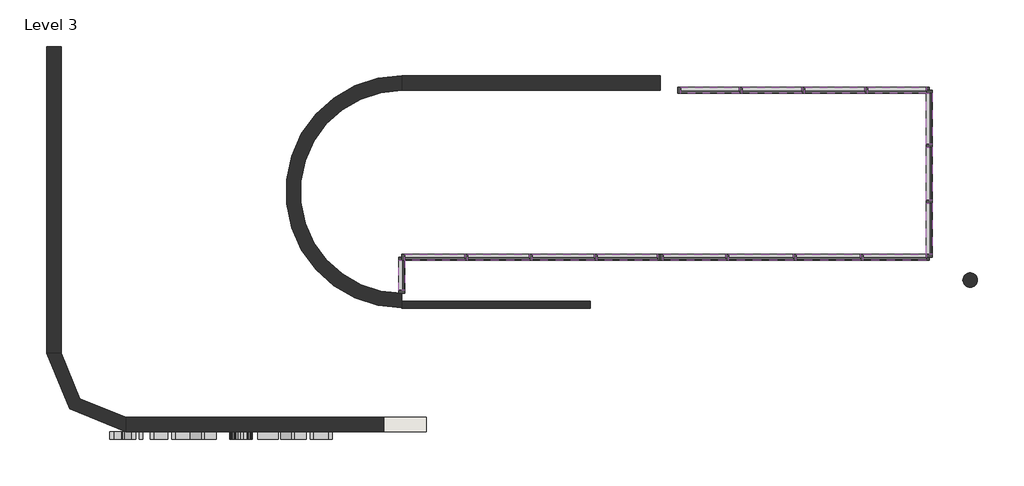
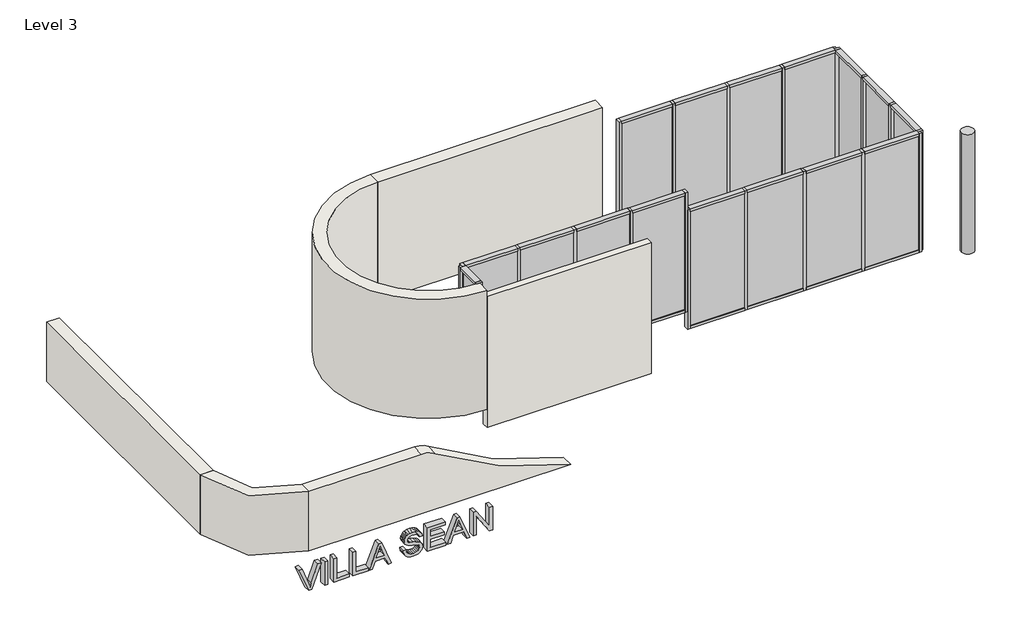
# One storey: 53 members, 16 plates, 6 walls, 1 column, 1 proxy.
"""IFC4 building model written with IfcOpenShell, lengths in millimetres."""

from ifc_helpers import new_model, si_unit, point, frame, frame_2d, origin, place, context, project, spatial, polyline, circle_curve, trimmed, segment, composite_curve, outline, extrude, transform, mapped, element, save
from components import column_6a8e800d, member_4d6ef9b1, member_8897803d, member_ef344e51, member_b14cf619, member_0d684f40, member_efa17701, member_5e365d0c, member_eaba9652, member_3f395ae9, member_5a365947, member_16d8dc0e, system_panel_glazed_93f0cbb4, system_panel_glazed_f623c012, system_panel_glazed_38c921e2, system_panel_glazed_90a2254b, system_panel_glazed_fd2dabf8, system_panel_glazed_5b6ff290, system_panel_glazed_14fb9695, system_panel_glazed_f99b9bb8, system_panel_glazed_f492b607

model = new_model("IFC4")

# Units and contexts
model_context = context("Model", 3, world=origin())
ifc_project = project(units=[si_unit("LENGTHUNIT", "METRE", prefix="MILLI")], contexts=[model_context])

# Site, building, storey
site = spatial("IfcSite", under=ifc_project)
building = spatial("IfcBuilding", under=site)
storey = spatial("IfcBuildingStorey", under=building, Name="Level 3", Elevation=6096.0)

# Proxy
placement = place(None, origin())
element("IfcBuildingElementProxy", 1, Name="24\" Arial", ObjectType="24\" Arial", at=placement, inside=storey, context=model_context, shape_type="SweptSolid", body=[
    extrude(outline(polyline([(6126.8228515, -15529.5610771), (6126.8228515, -15452.1887694), (6727.0443899, -15223.2956925), (6727.0443899, -15303.452231), (6294.6093899, -15463.7653079), (6197.161313, -15495.7106925), (6294.6093899, -15528.0956925), (6727.0443899, -15687.969154), (6727.0443899, -15768.272231), (6126.8228515, -15529.5610771)])), frame((0.0, 6721.4139644, 0.0), z_axis=(0.0, 1.0, 0.0), x_axis=(0.0, 0.0, 1.0)), (0.0, 0.0, 1.0), 152.4),
    extrude(outline(polyline([(-15068.9906925, 6721.4139644), (-15144.0183848, 6721.4139644), (-15144.0183848, 6873.8139644), (-15068.9906925, 6873.8139644), (-15068.9906925, 6721.4139644)])), frame((0.0, 0.0, 6126.8228515), z_axis=(0.0, 0.0, 1.0), x_axis=(1.0, 0.0, 0.0)), (0.0, 0.0, 1.0), 600.2215385),
    extrude(outline(polyline([(6126.8228515, -14918.9353079), (6126.8228515, -14543.7968463), (6201.8505438, -14543.7968463), (6201.8505438, -14843.9076156), (6727.0443899, -14843.9076156), (6727.0443899, -14918.9353079), (6126.8228515, -14918.9353079)])), frame((0.0, 6721.4139644, 0.0), z_axis=(0.0, 1.0, 0.0), x_axis=(0.0, 0.0, 1.0)), (0.0, 0.0, 1.0), 152.4),
    extrude(outline(polyline([(6126.8228515, -14459.3906925), (6126.8228515, -14084.252231), (6201.8505438, -14084.252231), (6201.8505438, -14384.3630002), (6727.0443899, -14384.3630002), (6727.0443899, -14459.3906925), (6126.8228515, -14459.3906925)])), frame((0.0, 6721.4139644, 0.0), z_axis=(0.0, 1.0, 0.0), x_axis=(0.0, 0.0, 1.0)), (0.0, 0.0, 1.0), 152.4),
    extrude(outline(polyline([(6126.8228515, -14069.5983848), (6126.8228515, -13990.4676156), (6314.3920822, -13921.8876156), (6314.3920822, -13674.5306925), (6126.8228515, -13605.9506925), (6126.8228515, -13526.6733848), (6727.0443899, -13766.117231), (6727.0443899, -13830.0080002), (6126.8228515, -14069.5983848)]), holes=[polyline([(6389.4197745, -13894.3383848), (6549.8793899, -13835.5764617), (6652.0166976, -13798.209154), (6536.9840053, -13756.1526156), (6389.4197745, -13701.9333848), (6389.4197745, -13894.3383848)])]), frame((0.0, 6721.4139644, 0.0), z_axis=(0.0, 1.0, 0.0), x_axis=(0.0, 0.0, 1.0)), (0.0, 0.0, 1.0), 152.4),
    extrude(outline(polyline([(6333.1490053, -13240.1906925), (6302.0278995, -13237.5621588), (6272.5553515, -13231.288481), (6244.7313611, -13221.3696588), (6218.5559284, -13207.8056925), (6194.7983803, -13190.9675074), (6174.2280438, -13171.226029), (6156.8449188, -13148.5812574), (6142.6490053, -13123.0331925), (6131.6219861, -13094.4078199), (6123.7455438, -13062.5311252), (6119.0196784, -13027.4031084), (6117.4443899, -12989.0237694), (6123.2876111, -12929.1444906), (6130.5916375, -12901.5540459), (6140.8172745, -12875.529731), (6153.6760245, -12851.7630242), (6168.8793899, -12830.945404), (6186.4273707, -12813.0768704), (6206.3199668, -12798.1574233), (6227.7283202, -12786.3931324), (6249.8235726, -12777.9900675), (6272.605724, -12772.9482286), (6296.0747745, -12771.2676156), (6341.3185245, -12777.1108367), (6361.8247505, -12784.4148632), (6380.9205438, -12794.6405002), (6398.5143178, -12807.9434449), (6414.5144861, -12824.4793944), (6441.7340053, -12867.2503079), (6459.2819861, -12917.2931925), (6479.3943899, -13000.014154), (6500.5691976, -13080.1706925), (6510.9917457, -13106.0713656), (6521.3043899, -13122.5203079), (6532.1940293, -13132.9703319), (6544.4941015, -13140.4346348), (6558.2046063, -13144.9132165), (6573.3255438, -13146.4060771), (6590.9010005, -13144.2995867), (6607.1392938, -13137.9801156), (6622.0404236, -13127.4476637), (6635.6043899, -13112.702231), (6646.8878515, -13093.3499954), (6654.9474668, -13068.9971348), (6659.7832361, -13039.6436492), (6661.3951591, -13005.2895387), (6659.7649188, -12971.9978319), (6654.8741976, -12943.0473271), (6646.7229957, -12918.4380242), (6635.311313, -12898.1699233), (6620.7124188, -12881.9407887), (6602.9995822, -12869.4483848), (6582.1728034, -12860.6927117), (6558.2320822, -12855.6737694), (6558.2320822, -12780.6460771), (6583.7755678, -12783.2746108), (6607.9452553, -12789.1086733), (6630.7411447, -12798.1482646), (6652.1632361, -12810.3933848), (6671.6436928, -12825.7249713), (6688.6146784, -12844.0239617), (6703.0761928, -12865.290356), (6715.0282361, -12889.524154), (6731.0741976, -12944.9156925), (6736.4228515, -13008.2203079), (6731.3123226, -13066.6525194), (6715.9807361, -13119.4430002), (6704.5690534, -13142.930368), (6690.7761207, -13163.422856), (6674.601938, -13180.9204641), (6656.0465053, -13195.4231925), (6635.9295221, -13206.8028199), (6615.070688, -13214.9311252), (6593.4700029, -13219.8081084), (6571.1274668, -13221.4337694), (6531.8185245, -13216.1767021), (6496.5393899, -13200.4055002), (6465.9494861, -13173.9369906), (6440.7082361, -13136.5880002), (6422.665688, -13090.7031444), (6403.7072745, -13018.9908848), (6375.0590053, -12909.7464617), (6359.5076111, -12877.7278079), (6340.988813, -12858.7510771), (6319.2828034, -12849.4092502), (6294.1697745, -12846.2953079), (6268.3973226, -12850.4533367), (6243.833813, -12862.9274233), (6222.4391976, -12883.9007406), (6206.1734284, -12913.5564617), (6195.8974188, -12950.1544425), (6192.4720822, -12991.9545387), (6196.9964572, -13039.4330002), (6210.5695822, -13081.929154), (6231.4879476, -13116.695404), (6258.0480438, -13140.984154), (6291.5137649, -13156.5538656), (6333.1490053, -13165.1630002), (6333.1490053, -13240.1906925)])), frame((0.0, 6721.4139644, 0.0), z_axis=(0.0, 1.0, 0.0), x_axis=(0.0, 0.0, 1.0)), (0.0, 0.0, 1.0), 152.4),
    extrude(outline(polyline([(6126.8228515, -12658.7260771), (6126.8228515, -12217.9383848), (6201.8505438, -12217.9383848), (6201.8505438, -12583.6983848), (6398.7982361, -12583.6983848), (6398.7982361, -12246.0737694), (6473.8259284, -12246.0737694), (6473.8259284, -12583.6983848), (6652.0166976, -12583.6983848), (6652.0166976, -12227.3168463), (6727.0443899, -12227.3168463), (6727.0443899, -12658.7260771), (6126.8228515, -12658.7260771)])), frame((0.0, 6721.4139644, 0.0), z_axis=(0.0, 1.0, 0.0), x_axis=(0.0, 0.0, 1.0)), (0.0, 0.0, 1.0), 152.4),
    extrude(outline(polyline([(6126.8228515, -12175.149154), (6126.8228515, -12096.0183848), (6314.3920822, -12027.4383848), (6314.3920822, -11780.0814617), (6126.8228515, -11711.5014617), (6126.8228515, -11632.224154), (6727.0443899, -11871.6680002), (6727.0443899, -11935.5587694), (6126.8228515, -12175.149154)]), holes=[polyline([(6389.4197745, -11999.889154), (6549.8793899, -11941.127231), (6652.0166976, -11903.7599233), (6536.9840053, -11861.7033848), (6389.4197745, -11807.484154), (6389.4197745, -11999.889154)])]), frame((0.0, 6721.4139644, 0.0), z_axis=(0.0, 1.0, 0.0), x_axis=(0.0, 0.0, 1.0)), (0.0, 0.0, 1.0), 152.4),
    extrude(outline(polyline([(6126.8228515, -11552.0676156), (6126.8228515, -11477.0399233), (6602.4866976, -11477.0399233), (6126.8228515, -11163.4476156), (6126.8228515, -11083.1445387), (6727.0443899, -11083.1445387), (6727.0443899, -11158.172231), (6251.5270822, -11158.172231), (6727.0443899, -11471.7645387), (6727.0443899, -11552.0676156), (6126.8228515, -11552.0676156)])), frame((0.0, 6721.4139644, 0.0), z_axis=(0.0, 1.0, 0.0), x_axis=(0.0, 0.0, 1.0)), (0.0, 0.0, 1.0), 152.4),
])

# Column
column_shape = column_6a8e800d(model_context)
element("IfcColumn", 2, ObjectType="Round Column.0002 : 06\" Diameter", at=placement, inside=storey, context=model_context, shape_type="MappedRepresentation", body=[
    mapped(column_shape, transform((-1667.0944013, 3216.2139644, 0.0), x_axis=(1.0, 0.0, 0.0), y_axis=(0.0, 1.0, 0.0), z_axis=(0.0, 0.0, 1.0))),
])

# Members
member_shape = member_4d6ef9b1(model_context)
element("IfcMember", 3, ObjectType="Rectangular Mullion : 2.5\" x 5\" rectangular", at=placement, inside=storey, context=model_context, shape_type="MappedRepresentation", body=[
    mapped(member_shape, transform((1468.8829427, 10615.9053975, 9601.2), x_axis=(0.0, 0.0, 1.0), y_axis=(-1.0, 0.0, 0.0), z_axis=(0.0, -1.0, 0.0))),
])
element("IfcMember", 4, ObjectType="Rectangular Mullion : 2.5\" x 5\" rectangular", at=placement, inside=storey, context=model_context, shape_type="MappedRepresentation", body=[
    mapped(member_shape, transform((1468.8829427, 12920.9553975, 9601.2), x_axis=(0.0, 0.0, 1.0), y_axis=(-1.0, 0.0, 0.0), z_axis=(0.0, -1.0, 0.0))),
])
member_2_shape = member_8897803d(model_context)
element("IfcMember", 5, ObjectType="Rectangular Mullion : 2.5\" x 5\" rectangular", at=placement, inside=storey, context=model_context, shape_type="MappedRepresentation", body=[
    mapped(member_2_shape, transform((1468.8829427, 11752.5553975, 9601.2), x_axis=(0.0, 0.0, 1.0), y_axis=(-1.0, 0.0, 0.0), z_axis=(0.0, -1.0, 0.0))),
])
element("IfcMember", 6, ObjectType="Rectangular Mullion : 2.5\" x 5\" rectangular", at=placement, inside=storey, context=model_context, shape_type="MappedRepresentation", body=[
    mapped(member_shape, transform((1468.8829427, 13994.1053975, 6553.2), x_axis=(0.0, 0.0, -1.0), y_axis=(-1.0, 0.0, 0.0), z_axis=(0.0, 1.0, 0.0))),
])
element("IfcMember", 7, ObjectType="Rectangular Mullion : 2.5\" x 5\" rectangular", at=placement, inside=storey, context=model_context, shape_type="MappedRepresentation", body=[
    mapped(member_shape, transform((1468.8829427, 11689.0553975, 6553.2), x_axis=(0.0, 0.0, -1.0), y_axis=(-1.0, 0.0, 0.0), z_axis=(0.0, 1.0, 0.0))),
])
element("IfcMember", 8, ObjectType="Rectangular Mullion : 2.5\" x 5\" rectangular", at=placement, inside=storey, context=model_context, shape_type="MappedRepresentation", body=[
    mapped(member_2_shape, transform((1468.8829427, 12857.4553975, 6553.2), x_axis=(0.0, 0.0, -1.0), y_axis=(-1.0, 0.0, 0.0), z_axis=(0.0, 1.0, 0.0))),
])
member_3_shape = member_ef344e51(model_context)
element("IfcMember", 9, ObjectType="Rectangular Mullion : 2.5\" x 5\" rectangular", at=placement, inside=storey, context=model_context, shape_type="MappedRepresentation", body=[
    mapped(member_3_shape, transform((-4128.3438771, 10552.4053975, 9601.2), x_axis=(0.0, 0.0, 1.0), y_axis=(0.0, 1.0, 0.0), z_axis=(-1.0, 0.0, 0.0))),
])
element("IfcMember", 10, ObjectType="Rectangular Mullion : 2.5\" x 5\" rectangular", at=placement, inside=storey, context=model_context, shape_type="MappedRepresentation", body=[
    mapped(member_3_shape, transform((85.4512378, 10552.4053975, 9601.2), x_axis=(0.0, 0.0, 1.0), y_axis=(0.0, 1.0, 0.0), z_axis=(-1.0, 0.0, 0.0))),
])
member_4_shape = member_b14cf619(model_context)
element("IfcMember", 11, ObjectType="Rectangular Mullion : 2.5\" x 5\" rectangular", at=placement, inside=storey, context=model_context, shape_type="MappedRepresentation", body=[
    mapped(member_4_shape, transform((-1329.7304672, 10552.4053975, 9601.2), x_axis=(0.0, 0.0, 1.0), y_axis=(0.0, 1.0, 0.0), z_axis=(-1.0, 0.0, 0.0))),
])
element("IfcMember", 12, ObjectType="Rectangular Mullion : 2.5\" x 5\" rectangular", at=placement, inside=storey, context=model_context, shape_type="MappedRepresentation", body=[
    mapped(member_4_shape, transform((-2744.9121722, 10552.4053975, 9601.2), x_axis=(0.0, 0.0, 1.0), y_axis=(0.0, 1.0, 0.0), z_axis=(-1.0, 0.0, 0.0))),
])
element("IfcMember", 13, ObjectType="Rectangular Mullion : 2.5\" x 5\" rectangular", at=placement, inside=storey, context=model_context, shape_type="MappedRepresentation", body=[
    mapped(member_3_shape, transform((1405.3829427, 10552.4053975, 6553.2), x_axis=(0.0, 0.0, -1.0), y_axis=(0.0, 1.0, 0.0), z_axis=(1.0, 0.0, 0.0))),
])
element("IfcMember", 14, ObjectType="Rectangular Mullion : 2.5\" x 5\" rectangular", at=placement, inside=storey, context=model_context, shape_type="MappedRepresentation", body=[
    mapped(member_3_shape, transform((-2808.4121722, 10552.4053975, 6553.2), x_axis=(0.0, 0.0, -1.0), y_axis=(0.0, 1.0, 0.0), z_axis=(1.0, 0.0, 0.0))),
])
element("IfcMember", 15, ObjectType="Rectangular Mullion : 2.5\" x 5\" rectangular", at=placement, inside=storey, context=model_context, shape_type="MappedRepresentation", body=[
    mapped(member_4_shape, transform((21.9512378, 10552.4053975, 6553.2), x_axis=(0.0, 0.0, -1.0), y_axis=(0.0, 1.0, 0.0), z_axis=(1.0, 0.0, 0.0))),
])
element("IfcMember", 16, ObjectType="Rectangular Mullion : 2.5\" x 5\" rectangular", at=placement, inside=storey, context=model_context, shape_type="MappedRepresentation", body=[
    mapped(member_4_shape, transform((-1393.2304672, 10552.4053975, 6553.2), x_axis=(0.0, 0.0, -1.0), y_axis=(0.0, 1.0, 0.0), z_axis=(1.0, 0.0, 0.0))),
])
member_5_shape = member_0d684f40(model_context)
element("IfcMember", 17, ObjectType="Rectangular Mullion : 2.5\" x 5\" rectangular", at=placement, inside=storey, context=model_context, shape_type="MappedRepresentation", body=[
    mapped(member_5_shape, transform((-9560.164807, 10552.4053975, 10058.4), x_axis=(0.0, 0.0, 1.0), y_axis=(0.0, 1.0, 0.0), z_axis=(-1.0, 0.0, 0.0))),
])
element("IfcMember", 18, ObjectType="Rectangular Mullion : 2.5\" x 5\" rectangular", at=placement, inside=storey, context=model_context, shape_type="MappedRepresentation", body=[
    mapped(member_5_shape, transform((-5518.0491096, 10552.4053975, 10058.4), x_axis=(0.0, 0.0, 1.0), y_axis=(0.0, 1.0, 0.0), z_axis=(-1.0, 0.0, 0.0))),
])
member_6_shape = member_efa17701(model_context)
element("IfcMember", 19, ObjectType="Rectangular Mullion : 2.5\" x 5\" rectangular", at=placement, inside=storey, context=model_context, shape_type="MappedRepresentation", body=[
    mapped(member_6_shape, transform((-6876.004342, 10552.4053975, 10058.4), x_axis=(0.0, 0.0, 1.0), y_axis=(0.0, 1.0, 0.0), z_axis=(-1.0, 0.0, 0.0))),
])
element("IfcMember", 20, ObjectType="Rectangular Mullion : 2.5\" x 5\" rectangular", at=placement, inside=storey, context=model_context, shape_type="MappedRepresentation", body=[
    mapped(member_6_shape, transform((-8233.9595745, 10552.4053975, 10058.4), x_axis=(0.0, 0.0, 1.0), y_axis=(0.0, 1.0, 0.0), z_axis=(-1.0, 0.0, 0.0))),
])
element("IfcMember", 21, ObjectType="Rectangular Mullion : 2.5\" x 5\" rectangular", at=placement, inside=storey, context=model_context, shape_type="MappedRepresentation", body=[
    mapped(member_5_shape, transform((-4255.3438771, 10552.4053975, 7010.4), x_axis=(0.0, 0.0, -1.0), y_axis=(0.0, 1.0, 0.0), z_axis=(1.0, 0.0, 0.0))),
])
element("IfcMember", 22, ObjectType="Rectangular Mullion : 2.5\" x 5\" rectangular", at=placement, inside=storey, context=model_context, shape_type="MappedRepresentation", body=[
    mapped(member_5_shape, transform((-8297.4595745, 10552.4053975, 7010.4), x_axis=(0.0, 0.0, -1.0), y_axis=(0.0, 1.0, 0.0), z_axis=(1.0, 0.0, 0.0))),
])
element("IfcMember", 23, ObjectType="Rectangular Mullion : 2.5\" x 5\" rectangular", at=placement, inside=storey, context=model_context, shape_type="MappedRepresentation", body=[
    mapped(member_6_shape, transform((-5581.5491096, 10552.4053975, 7010.4), x_axis=(0.0, 0.0, -1.0), y_axis=(0.0, 1.0, 0.0), z_axis=(1.0, 0.0, 0.0))),
])
element("IfcMember", 24, ObjectType="Rectangular Mullion : 2.5\" x 5\" rectangular", at=placement, inside=storey, context=model_context, shape_type="MappedRepresentation", body=[
    mapped(member_6_shape, transform((-6939.504342, 10552.4053975, 7010.4), x_axis=(0.0, 0.0, -1.0), y_axis=(0.0, 1.0, 0.0), z_axis=(1.0, 0.0, 0.0))),
])
member_7_shape = member_5e365d0c(model_context)
element("IfcMember", 25, ObjectType="Rectangular Mullion : 2.5\" x 5\" rectangular", at=placement, inside=storey, context=model_context, shape_type="MappedRepresentation", body=[
    mapped(member_7_shape, transform((-9623.664807, 9853.9053975, 10058.4), x_axis=(0.0, 0.0, 1.0), y_axis=(-1.0, 0.0, 0.0), z_axis=(0.0, -1.0, 0.0))),
])
element("IfcMember", 26, ObjectType="Rectangular Mullion : 2.5\" x 5\" rectangular", at=placement, inside=storey, context=model_context, shape_type="MappedRepresentation", body=[
    mapped(member_7_shape, transform((-9623.664807, 10488.9053975, 7010.4), x_axis=(0.0, 0.0, -1.0), y_axis=(-1.0, 0.0, 0.0), z_axis=(0.0, 1.0, 0.0))),
])
member_8_shape = member_eaba9652(model_context)
element("IfcMember", 27, ObjectType="Rectangular Mullion : 2.5\" x 5\" rectangular", at=placement, inside=storey, context=model_context, shape_type="MappedRepresentation", body=[
    mapped(member_8_shape, transform((1468.8829427, 12889.2053975, 6553.2), x_axis=(0.0, -1.0, 0.0), y_axis=(-1.0, 0.0, 0.0), z_axis=(0.0, 0.0, -1.0))),
])
element("IfcMember", 28, ObjectType="Rectangular Mullion : 2.5\" x 5\" rectangular", at=placement, inside=storey, context=model_context, shape_type="MappedRepresentation", body=[
    mapped(member_8_shape, transform((1468.8829427, 11720.8053975, 6553.2), x_axis=(0.0, -1.0, 0.0), y_axis=(-1.0, 0.0, 0.0), z_axis=(0.0, 0.0, -1.0))),
])
element("IfcMember", 29, ObjectType="Rectangular Mullion : 2.5\" x 5\" rectangular", at=placement, inside=storey, context=model_context, shape_type="MappedRepresentation", body=[
    mapped(member_8_shape, transform((53.7012378, 10552.4053975, 6553.2), x_axis=(-1.0, 0.0, 0.0), y_axis=(0.0, 1.0, 0.0), z_axis=(0.0, 0.0, -1.0))),
])
element("IfcMember", 30, ObjectType="Rectangular Mullion : 2.5\" x 5\" rectangular", at=placement, inside=storey, context=model_context, shape_type="MappedRepresentation", body=[
    mapped(member_8_shape, transform((-1361.4804672, 10552.4053975, 6553.2), x_axis=(-1.0, 0.0, 0.0), y_axis=(0.0, 1.0, 0.0), z_axis=(0.0, 0.0, -1.0))),
])
element("IfcMember", 31, ObjectType="Rectangular Mullion : 2.5\" x 5\" rectangular", at=placement, inside=storey, context=model_context, shape_type="MappedRepresentation", body=[
    mapped(member_8_shape, transform((-2776.6621722, 10552.4053975, 6553.2), x_axis=(-1.0, 0.0, 0.0), y_axis=(0.0, 1.0, 0.0), z_axis=(0.0, 0.0, -1.0))),
])
element("IfcMember", 32, ObjectType="Rectangular Mullion : 2.5\" x 5\" rectangular", at=placement, inside=storey, context=model_context, shape_type="MappedRepresentation", body=[
    mapped(member_8_shape, transform((-5549.7991096, 10552.4053975, 7010.4), x_axis=(-1.0, 0.0, 0.0), y_axis=(0.0, 1.0, 0.0), z_axis=(0.0, 0.0, -1.0))),
])
element("IfcMember", 33, ObjectType="Rectangular Mullion : 2.5\" x 5\" rectangular", at=placement, inside=storey, context=model_context, shape_type="MappedRepresentation", body=[
    mapped(member_8_shape, transform((-6907.754342, 10552.4053975, 7010.4), x_axis=(-1.0, 0.0, 0.0), y_axis=(0.0, 1.0, 0.0), z_axis=(0.0, 0.0, -1.0))),
])
element("IfcMember", 34, ObjectType="Rectangular Mullion : 2.5\" x 5\" rectangular", at=placement, inside=storey, context=model_context, shape_type="MappedRepresentation", body=[
    mapped(member_8_shape, transform((-8265.7095745, 10552.4053975, 7010.4), x_axis=(-1.0, 0.0, 0.0), y_axis=(0.0, 1.0, 0.0), z_axis=(0.0, 0.0, -1.0))),
])
element("IfcMember", 35, ObjectType="Rectangular Mullion : 2.5\" x 5\" rectangular", at=placement, inside=storey, context=model_context, shape_type="MappedRepresentation", body=[
    mapped(member_8_shape, transform((146.0574827, 14057.6053975, 6553.2), x_axis=(-1.0, 0.0, 0.0), y_axis=(0.0, 1.0, 0.0), z_axis=(0.0, 0.0, -1.0))),
])
element("IfcMember", 36, ObjectType="Rectangular Mullion : 2.5\" x 5\" rectangular", at=placement, inside=storey, context=model_context, shape_type="MappedRepresentation", body=[
    mapped(member_8_shape, transform((-1176.7679772, 14057.6053975, 6553.2), x_axis=(-1.0, 0.0, 0.0), y_axis=(0.0, 1.0, 0.0), z_axis=(0.0, 0.0, -1.0))),
])
element("IfcMember", 37, ObjectType="Rectangular Mullion : 2.5\" x 5\" rectangular", at=placement, inside=storey, context=model_context, shape_type="MappedRepresentation", body=[
    mapped(member_8_shape, transform((-2499.5934372, 14057.6053975, 6553.2), x_axis=(-1.0, 0.0, 0.0), y_axis=(0.0, 1.0, 0.0), z_axis=(0.0, 0.0, -1.0))),
])
member_9_shape = member_3f395ae9(model_context)
element("IfcMember", 38, ObjectType="Rectangular Mullion : 2.5\" x 5\" rectangular", at=placement, inside=storey, context=model_context, shape_type="MappedRepresentation", body=[
    mapped(member_9_shape, transform((1468.8829427, 10552.4053975, 6553.2), x_axis=(0.0, -1.0, 0.0), y_axis=(-1.0, 0.0, 0.0), z_axis=(0.0, 0.0, -1.0))),
])
element("IfcMember", 39, ObjectType="Rectangular Mullion : 2.5\" x 5\" rectangular", at=placement, inside=storey, context=model_context, shape_type="MappedRepresentation", body=[
    mapped(member_9_shape, transform((-4191.8438771, 10552.4053975, 6553.2), x_axis=(-1.0, 0.0, 0.0), y_axis=(0.0, 1.0, 0.0), z_axis=(0.0, 0.0, -1.0))),
])
element("IfcMember", 40, ObjectType="Rectangular Mullion : 2.5\" x 5\" rectangular", at=placement, inside=storey, context=model_context, shape_type="MappedRepresentation", body=[
    mapped(member_9_shape, transform((-9623.664807, 10552.4053975, 7010.4), x_axis=(-1.0, 0.0, 0.0), y_axis=(0.0, 1.0, 0.0), z_axis=(0.0, 0.0, -1.0))),
])
element("IfcMember", 41, ObjectType="Rectangular Mullion : 2.5\" x 5\" rectangular", at=placement, inside=storey, context=model_context, shape_type="MappedRepresentation", body=[
    mapped(member_9_shape, transform((-9623.664807, 9790.4053975, 7010.4), x_axis=(0.0, -1.0, 0.0), y_axis=(-1.0, 0.0, 0.0), z_axis=(0.0, 0.0, -1.0))),
])
element("IfcMember", 42, ObjectType="Rectangular Mullion : 2.5\" x 5\" rectangular", at=placement, inside=storey, context=model_context, shape_type="MappedRepresentation", body=[
    mapped(member_9_shape, transform((-3822.4188972, 14057.6053975, 6553.2), x_axis=(-1.0, 0.0, 0.0), y_axis=(0.0, 1.0, 0.0), z_axis=(0.0, 0.0, -1.0))),
])
element("IfcMember", 43, ObjectType="Rectangular Mullion : 2.5\" x 5\" rectangular", at=placement, inside=storey, context=model_context, shape_type="MappedRepresentation", body=[
    mapped(member_9_shape, transform((1468.8829427, 14057.6053975, 9601.2), x_axis=(0.0, 1.0, 0.0), y_axis=(-1.0, 0.0, 0.0), z_axis=(0.0, 0.0, 1.0))),
])
element("IfcMember", 44, ObjectType="Rectangular Mullion : 2.5\" x 5\" rectangular", at=placement, inside=storey, context=model_context, shape_type="MappedRepresentation", body=[
    mapped(member_9_shape, transform((1468.8829427, 10552.4053975, 9601.2), x_axis=(1.0, 0.0, 0.0), y_axis=(0.0, 1.0, 0.0), z_axis=(0.0, 0.0, 1.0))),
])
element("IfcMember", 45, ObjectType="Rectangular Mullion : 2.5\" x 5\" rectangular", at=placement, inside=storey, context=model_context, shape_type="MappedRepresentation", body=[
    mapped(member_9_shape, transform((-4191.8438771, 10552.4053975, 10058.4), x_axis=(1.0, 0.0, 0.0), y_axis=(0.0, 1.0, 0.0), z_axis=(0.0, 0.0, 1.0))),
])
element("IfcMember", 46, ObjectType="Rectangular Mullion : 2.5\" x 5\" rectangular", at=placement, inside=storey, context=model_context, shape_type="MappedRepresentation", body=[
    mapped(member_9_shape, transform((-9623.664807, 10552.4053975, 10058.4), x_axis=(0.0, 1.0, 0.0), y_axis=(-1.0, 0.0, 0.0), z_axis=(0.0, 0.0, 1.0))),
])
element("IfcMember", 47, ObjectType="Rectangular Mullion : 2.5\" x 5\" rectangular", at=placement, inside=storey, context=model_context, shape_type="MappedRepresentation", body=[
    mapped(member_9_shape, transform((1468.8829427, 14057.6053975, 9601.2), x_axis=(1.0, 0.0, 0.0), y_axis=(0.0, 1.0, 0.0), z_axis=(0.0, 0.0, 1.0))),
])
member_10_shape = member_5a365947(model_context)
element("IfcMember", 48, ObjectType="Rectangular Mullion : 2.5\" x 5\" rectangular", at=placement, inside=storey, context=model_context, shape_type="MappedRepresentation", body=[
    mapped(member_10_shape, transform((-3758.9188972, 14057.6053975, 9601.2), x_axis=(0.0, 0.0, 1.0), y_axis=(0.0, 1.0, 0.0), z_axis=(-1.0, 0.0, 0.0))),
])
element("IfcMember", 49, ObjectType="Rectangular Mullion : 2.5\" x 5\" rectangular", at=placement, inside=storey, context=model_context, shape_type="MappedRepresentation", body=[
    mapped(member_10_shape, transform((177.8074827, 14057.6053975, 9601.2), x_axis=(0.0, 0.0, 1.0), y_axis=(0.0, 1.0, 0.0), z_axis=(-1.0, 0.0, 0.0))),
])
member_11_shape = member_16d8dc0e(model_context)
element("IfcMember", 50, ObjectType="Rectangular Mullion : 2.5\" x 5\" rectangular", at=placement, inside=storey, context=model_context, shape_type="MappedRepresentation", body=[
    mapped(member_11_shape, transform((-1145.0179772, 14057.6053975, 9601.2), x_axis=(0.0, 0.0, 1.0), y_axis=(0.0, 1.0, 0.0), z_axis=(-1.0, 0.0, 0.0))),
])
element("IfcMember", 51, ObjectType="Rectangular Mullion : 2.5\" x 5\" rectangular", at=placement, inside=storey, context=model_context, shape_type="MappedRepresentation", body=[
    mapped(member_11_shape, transform((-2467.8434372, 14057.6053975, 9601.2), x_axis=(0.0, 0.0, 1.0), y_axis=(0.0, 1.0, 0.0), z_axis=(-1.0, 0.0, 0.0))),
])
element("IfcMember", 52, ObjectType="Rectangular Mullion : 2.5\" x 5\" rectangular", at=placement, inside=storey, context=model_context, shape_type="MappedRepresentation", body=[
    mapped(member_10_shape, transform((1405.3829427, 14057.6053975, 6553.2), x_axis=(0.0, 0.0, -1.0), y_axis=(0.0, 1.0, 0.0), z_axis=(1.0, 0.0, 0.0))),
])
element("IfcMember", 53, ObjectType="Rectangular Mullion : 2.5\" x 5\" rectangular", at=placement, inside=storey, context=model_context, shape_type="MappedRepresentation", body=[
    mapped(member_10_shape, transform((-2531.3434372, 14057.6053975, 6553.2), x_axis=(0.0, 0.0, -1.0), y_axis=(0.0, 1.0, 0.0), z_axis=(1.0, 0.0, 0.0))),
])
element("IfcMember", 54, ObjectType="Rectangular Mullion : 2.5\" x 5\" rectangular", at=placement, inside=storey, context=model_context, shape_type="MappedRepresentation", body=[
    mapped(member_11_shape, transform((114.3074827, 14057.6053975, 6553.2), x_axis=(0.0, 0.0, -1.0), y_axis=(0.0, 1.0, 0.0), z_axis=(1.0, 0.0, 0.0))),
])
element("IfcMember", 55, ObjectType="Rectangular Mullion : 2.5\" x 5\" rectangular", at=placement, inside=storey, context=model_context, shape_type="MappedRepresentation", body=[
    mapped(member_11_shape, transform((-1208.5179772, 14057.6053975, 6553.2), x_axis=(0.0, 0.0, -1.0), y_axis=(0.0, 1.0, 0.0), z_axis=(1.0, 0.0, 0.0))),
])

# Plates
system_panel_glazed_shape = system_panel_glazed_93f0cbb4(model_context)
element("IfcPlate", 56, ObjectType="System Panel : Glazed", at=placement, inside=storey, context=model_context, shape_type="MappedRepresentation", body=[
    mapped(system_panel_glazed_shape, transform((745.4170902, 10552.4053975, 6616.7), x_axis=(-1.0, 0.0, 0.0), y_axis=(0.0, -1.0, 0.0), z_axis=(0.0, 0.0, 1.0))),
])
element("IfcPlate", 57, ObjectType="System Panel : Glazed", at=placement, inside=storey, context=model_context, shape_type="MappedRepresentation", body=[
    mapped(system_panel_glazed_shape, transform((-3468.3780246, 10552.4053975, 6616.7), x_axis=(-1.0, 0.0, 0.0), y_axis=(0.0, -1.0, 0.0), z_axis=(0.0, 0.0, 1.0))),
])
system_panel_glazed_2_shape = system_panel_glazed_f623c012(model_context)
element("IfcPlate", 58, ObjectType="System Panel : Glazed", at=placement, inside=storey, context=model_context, shape_type="MappedRepresentation", body=[
    mapped(system_panel_glazed_2_shape, transform((-653.8896147, 10552.4053975, 6616.7), x_axis=(-1.0, 0.0, 0.0), y_axis=(0.0, -1.0, 0.0), z_axis=(0.0, 0.0, 1.0))),
])
element("IfcPlate", 59, ObjectType="System Panel : Glazed", at=placement, inside=storey, context=model_context, shape_type="MappedRepresentation", body=[
    mapped(system_panel_glazed_2_shape, transform((-2069.0713197, 10552.4053975, 6616.7), x_axis=(-1.0, 0.0, 0.0), y_axis=(0.0, -1.0, 0.0), z_axis=(0.0, 0.0, 1.0))),
])
system_panel_glazed_3_shape = system_panel_glazed_38c921e2(model_context)
element("IfcPlate", 60, ObjectType="System Panel : Glazed", at=placement, inside=storey, context=model_context, shape_type="MappedRepresentation", body=[
    mapped(system_panel_glazed_3_shape, transform((1468.8829427, 13457.5303975, 6616.7), x_axis=(0.0, -1.0, 0.0), y_axis=(1.0, 0.0, 0.0), z_axis=(0.0, 0.0, 1.0))),
])
element("IfcPlate", 61, ObjectType="System Panel : Glazed", at=placement, inside=storey, context=model_context, shape_type="MappedRepresentation", body=[
    mapped(system_panel_glazed_3_shape, transform((1468.8829427, 11152.4803975, 6616.7), x_axis=(0.0, -1.0, 0.0), y_axis=(1.0, 0.0, 0.0), z_axis=(0.0, 0.0, 1.0))),
])
system_panel_glazed_4_shape = system_panel_glazed_90a2254b(model_context)
element("IfcPlate", 62, ObjectType="System Panel : Glazed", at=placement, inside=storey, context=model_context, shape_type="MappedRepresentation", body=[
    mapped(system_panel_glazed_4_shape, transform((1468.8829427, 12305.0053975, 6616.7), x_axis=(0.0, -1.0, 0.0), y_axis=(1.0, 0.0, 0.0), z_axis=(0.0, 0.0, 1.0))),
])
system_panel_glazed_5_shape = system_panel_glazed_fd2dabf8(model_context)
element("IfcPlate", 63, ObjectType="System Panel : Glazed", at=placement, inside=storey, context=model_context, shape_type="MappedRepresentation", body=[
    mapped(system_panel_glazed_5_shape, transform((-4886.6964933, 10552.4053975, 7073.9), x_axis=(-1.0, 0.0, 0.0), y_axis=(0.0, -1.0, 0.0), z_axis=(0.0, 0.0, 1.0))),
])
element("IfcPlate", 64, ObjectType="System Panel : Glazed", at=placement, inside=storey, context=model_context, shape_type="MappedRepresentation", body=[
    mapped(system_panel_glazed_5_shape, transform((-8928.8121907, 10552.4053975, 7073.9), x_axis=(-1.0, 0.0, 0.0), y_axis=(0.0, -1.0, 0.0), z_axis=(0.0, 0.0, 1.0))),
])
system_panel_glazed_6_shape = system_panel_glazed_5b6ff290(model_context)
element("IfcPlate", 65, ObjectType="System Panel : Glazed", at=placement, inside=storey, context=model_context, shape_type="MappedRepresentation", body=[
    mapped(system_panel_glazed_6_shape, transform((-6228.7767258, 10552.4053975, 7073.9), x_axis=(-1.0, 0.0, 0.0), y_axis=(0.0, -1.0, 0.0), z_axis=(0.0, 0.0, 1.0))),
])
element("IfcPlate", 66, ObjectType="System Panel : Glazed", at=placement, inside=storey, context=model_context, shape_type="MappedRepresentation", body=[
    mapped(system_panel_glazed_6_shape, transform((-7586.7319583, 10552.4053975, 7073.9), x_axis=(-1.0, 0.0, 0.0), y_axis=(0.0, -1.0, 0.0), z_axis=(0.0, 0.0, 1.0))),
])
system_panel_glazed_7_shape = system_panel_glazed_14fb9695(model_context)
element("IfcPlate", 67, ObjectType="System Panel : Glazed", at=placement, inside=storey, context=model_context, shape_type="MappedRepresentation", body=[
    mapped(system_panel_glazed_7_shape, transform((-9623.664807, 10171.4053975, 7073.9), x_axis=(0.0, -1.0, 0.0), y_axis=(1.0, 0.0, 0.0), z_axis=(0.0, 0.0, 1.0))),
])
system_panel_glazed_8_shape = system_panel_glazed_f99b9bb8(model_context)
element("IfcPlate", 68, ObjectType="System Panel : Glazed", at=placement, inside=storey, context=model_context, shape_type="MappedRepresentation", body=[
    mapped(system_panel_glazed_8_shape, transform((791.5952127, 14057.6053975, 6616.7), x_axis=(-1.0, 0.0, 0.0), y_axis=(0.0, -1.0, 0.0), z_axis=(0.0, 0.0, 1.0))),
])
element("IfcPlate", 69, ObjectType="System Panel : Glazed", at=placement, inside=storey, context=model_context, shape_type="MappedRepresentation", body=[
    mapped(system_panel_glazed_8_shape, transform((-3145.1311672, 14057.6053975, 6616.7), x_axis=(-1.0, 0.0, 0.0), y_axis=(0.0, -1.0, 0.0), z_axis=(0.0, 0.0, 1.0))),
])
system_panel_glazed_9_shape = system_panel_glazed_f492b607(model_context)
element("IfcPlate", 70, ObjectType="System Panel : Glazed", at=placement, inside=storey, context=model_context, shape_type="MappedRepresentation", body=[
    mapped(system_panel_glazed_9_shape, transform((-515.3552472, 14057.6053975, 6616.7), x_axis=(-1.0, 0.0, 0.0), y_axis=(0.0, -1.0, 0.0), z_axis=(0.0, 0.0, 1.0))),
])
element("IfcPlate", 71, ObjectType="System Panel : Glazed", at=placement, inside=storey, context=model_context, shape_type="MappedRepresentation", body=[
    mapped(system_panel_glazed_9_shape, transform((-1838.1807072, 14057.6053975, 6616.7), x_axis=(-1.0, 0.0, 0.0), y_axis=(0.0, -1.0, 0.0), z_axis=(0.0, 0.0, 1.0))),
])

# Walls
element("IfcWall", 72, ObjectType="Generic - 12\" white", at=placement, inside=storey, context=model_context, shape_type="SweptSolid", body=[
    extrude(outline(composite_curve([segment(polyline([(7010.4, -15435.2693346), (7010.4, -9106.3035766)]), True, "CONTINUOUS"), segment(trimmed(circle_curve(frame_2d((16065.0645611, -7113.6731034)), 9271.328196), [point((7010.4, -9106.3035766))], [point((8425.0739731, -12366.1078086))], True, "CARTESIAN"), True, "CONTINUOUS"), segment(trimmed(circle_curve(frame_2d((7915.1188189, -12717.4693346)), 619.2811811), [point((8425.0739731, -12366.1078086))], [point((8534.4, -12717.4693346))], False, "CARTESIAN"), True, "CONTINUOUS"), segment(polyline([(8534.4, -12717.4693346), (8534.4, -15435.2693346), (7010.4, -15435.2693346)]), True, "CONTINUOUS")], self_intersect=False)), frame((0.0, 6873.8139644, 0.0), z_axis=(0.0, 1.0, 0.0), x_axis=(0.0, 0.0, 1.0)), (0.0, 0.0, 1.0), 304.8),
])
element("IfcWall", 73, ObjectType="Generic - 12\" white", at=placement, inside=storey, context=model_context, shape_type="SweptSolid", body=[
    extrude(outline(composite_curve([segment(polyline([(-17096.3523629, 8534.8969927), (-16791.5523629, 8534.8969927)]), True, "CONTINUOUS"), segment(trimmed(circle_curve(frame_2d((-15435.2693346, 8534.8969927)), 1356.2830283), [point((-16791.5523629, 8534.8969927))], [point((-15435.2693346, 7178.6139644))], True, "CARTESIAN"), True, "CONTINUOUS"), segment(polyline([(-15435.2693346, 7178.6139644), (-15435.2693346, 6873.8139644)]), True, "CONTINUOUS"), segment(trimmed(circle_curve(frame_2d((-15435.2693346, 8534.8969927)), 1661.0830283), [point((-15435.2693346, 6873.8139644))], [point((-17096.3523629, 8534.8969927))], False, "CARTESIAN"), True, "CONTINUOUS")], self_intersect=False)), frame((0.0, 0.0, 7010.4), z_axis=(0.0, 0.0, 1.0), x_axis=(1.0, 0.0, 0.0)), (0.0, 0.0, 1.0), 1524.0),
])
element("IfcWall", 74, ObjectType="Generic - 12\" white", at=placement, inside=storey, context=model_context, shape_type="SweptSolid", body=[
    extrude(outline(polyline([(-16791.5523629, 14980.6629979), (-16791.5523629, 8534.8969927), (-17096.3523629, 8534.8969927), (-17096.3523629, 14980.6629979), (-16791.5523629, 14980.6629979)])), frame((0.0, 0.0, 7010.4), z_axis=(0.0, 0.0, 1.0), x_axis=(1.0, 0.0, 0.0)), (0.0, 0.0, 1.0), 1524.0),
])
element("IfcWall", 75, ObjectType="Generic - 12\" white", at=placement, inside=storey, context=model_context, shape_type="SweptSolid", body=[
    extrude(outline(composite_curve([segment(polyline([(-9623.664807, 14362.4053975), (-9623.664807, 14057.6053975)]), True, "CONTINUOUS"), segment(trimmed(circle_curve(frame_2d((-9623.664807, 11924.0053975)), 2133.6), [point((-9623.664807, 14057.6053975))], [point((-9623.664807, 9790.4053975))], True, "CARTESIAN"), True, "CONTINUOUS"), segment(polyline([(-9623.664807, 9790.4053975), (-9623.664807, 9485.6053975)]), True, "CONTINUOUS"), segment(trimmed(circle_curve(frame_2d((-9623.664807, 11924.0053975)), 2438.4), [point((-9623.664807, 9485.6053975))], [point((-9623.664807, 14362.4053975))], False, "CARTESIAN"), True, "CONTINUOUS")], self_intersect=False)), frame((0.0, 0.0, 7010.4), z_axis=(0.0, 0.0, 1.0), x_axis=(1.0, 0.0, 0.0)), (0.0, 0.0, 1.0), 3048.0),
])
element("IfcWall", 76, ObjectType="Generic - 12\" white", at=placement, inside=storey, context=model_context, shape_type="SweptSolid", body=[
    extrude(outline(polyline([(-4191.8438771, 14057.6053975), (-9623.664807, 14057.6053975), (-9623.664807, 14362.4053975), (-4191.8438771, 14362.4053975), (-4191.8438771, 14057.6053975)])), frame((0.0, 0.0, 7010.4), z_axis=(0.0, 0.0, 1.0), x_axis=(1.0, 0.0, 0.0)), (0.0, 0.0, 1.0), 3048.0),
])
element("IfcWall", 77, ObjectType="Generic - 6\" brown", at=placement, inside=storey, context=model_context, shape_type="SweptSolid", body=[
    extrude(outline(polyline([(-5661.264807, 9475.8209117), (-9623.664807, 9475.8209117), (-9623.664807, 9628.2209117), (-5661.264807, 9628.2209117), (-5661.264807, 9475.8209117)])), frame((0.0, 0.0, 6553.2), z_axis=(0.0, 0.0, 1.0), x_axis=(1.0, 0.0, 0.0)), (0.0, 0.0, 1.0), 3352.8),
])

save(model, "model.ifc")

# Revit data of these elements
# Type "Round Column.0002 : 06\" Diameter"
#   Assembly Code = "B1010200"
#   Diameter = 0' - 6"
#   Offset Base = 0' - 0"
#   Offset Top = 0' - 0"
#   Material = none
# Type "Rectangular Mullion : 2.5\" x 5\" rectangular"
#   built-in parameter 1007304 = 0.416667 (stored number, unit not read)
#   built-in parameter 1007301 = 0.104167 (stored number, unit not read)
#   built-in parameter 1007300 = 0.104167 (stored number, unit not read)
# Type "System Panel : Glazed"
#   Construction Type Id = "GSP4R"
#   Analytic Construction = "1/8 in Pilkington single glazing"
#   Visual Light Transmittance = 0.9
#   Solar Heat Gain Coefficient = 0.86
#   Heat Transfer Coefficient (U) = 1.18115 BTU/(h·ft²·°F)
# Type "Generic - 12\" white"
#   Assembly Code = "B2010"
#   Layers, outside or top first: 1' - 0" "Door - Frame" (function 1)
# Type "Generic - 6\" brown"
#   Assembly Code = "B2010"
#   Layers, outside or top first: 0' - 6" "Door - Panel" (function 1)
# Element 1 (IfcBuildingElementProxy, "24\" Arial")
#   Phase Created = New Construction
# Element 2 (IfcColumn, "Round Column.0002 : 06\" Diameter")
#   Phase Created = New Construction
# Elements 3, 4, 5, 6, 7, 8, 9, 10, 11, 12, 13, 14, 15, 16, 17, 18, 19, 20, 21, 22, 23, 24, 25, 26, 27, 28, 29, 30, 31, 32, 33, 34, 35, 36, 37, 38, 39, 40, 41, 42, 43, 44, 45, 46, 47, 48, 49, 50, 51, 52, 53, 54, 55 (IfcMember, "Rectangular Mullion : 2.5\" x 5\" rectangular")
#   Phase Created = New Construction
#   Materials on its faces: "Iron, Ductile"
# Elements 56, 57, 58, 59, 60, 61, 62, 63, 64, 65, 66, 67, 68, 69, 70, 71 (IfcPlate, "System Panel : Glazed")
#   Phase Created = New Construction
#   Materials on its faces: "Glass"
# Elements 72, 74 (IfcWall, "Generic - 12\" white")
#   built-in parameter 1001111 = 3' - 0"
#   Top Offset = 0' - 0"
#   Base Offset = 3' - 0"
#   Unconnected Height = 5' - 0"
#   wall height = 5' - 0"
#   Phase Created = New Construction
#   Base Constraint = Level 3
#   Materials on its faces: "Door - Frame"
# Element 73 (IfcWall, "Generic - 12\" white")
#   built-in parameter 1001111 = 3' - 0"
#   Top Offset = 0' - 0"
#   Base Offset = 3' - 0"
#   Unconnected Height = 5' - 0"
#   wall height = 5' - 0"
#   Phase Created = New Construction
#   Materials on its faces: "Door - Frame"
# Element 75 (IfcWall, "Generic - 12\" white")
#   built-in parameter 1001111 = 3' - 0"
#   Top Offset = 0' - 0"
#   Base Offset = 3' - 0"
#   Unconnected Height = 10' - 0"
#   wall height = 10' - 0"
#   Phase Created = New Construction
#   Materials on its faces: "Door - Frame"
# Element 76 (IfcWall, "Generic - 12\" white")
#   built-in parameter 1001111 = 3' - 0"
#   Top Offset = 0' - 0"
#   Base Offset = 3' - 0"
#   Unconnected Height = 10' - 0"
#   wall height = 10' - 0"
#   Phase Created = New Construction
#   Base Constraint = Level 3
#   Materials on its faces: "Door - Frame"
# Element 77 (IfcWall, "Generic - 6\" brown")
#   built-in parameter 1001111 = 1' - 6"
#   Top Offset = 0' - 0"
#   Base Offset = 1' - 6"
#   Unconnected Height = 11' - 0"
#   wall height = 11' - 0"
#   Phase Created = New Construction
#   Base Constraint = Level 3
#   Materials on its faces: "Door - Panel"
# Materials
#   "Door - Frame": colour RGB 118 70 51, transparency 0, Cost = 0
#   "Door - Panel": class "Wood", colour RGB 210 159 95, transparency 0, Cost = 0
#   "Iron, Ductile": class "Metal", colour RGB 0 0 0, transparency 0, Description = "Ductile cast iron", Cost = 0
#   "Glass": class "Glass", colour RGB 0 128 192, transparency 0.75, Description = "Soda Lime Glass", Cost = 0
